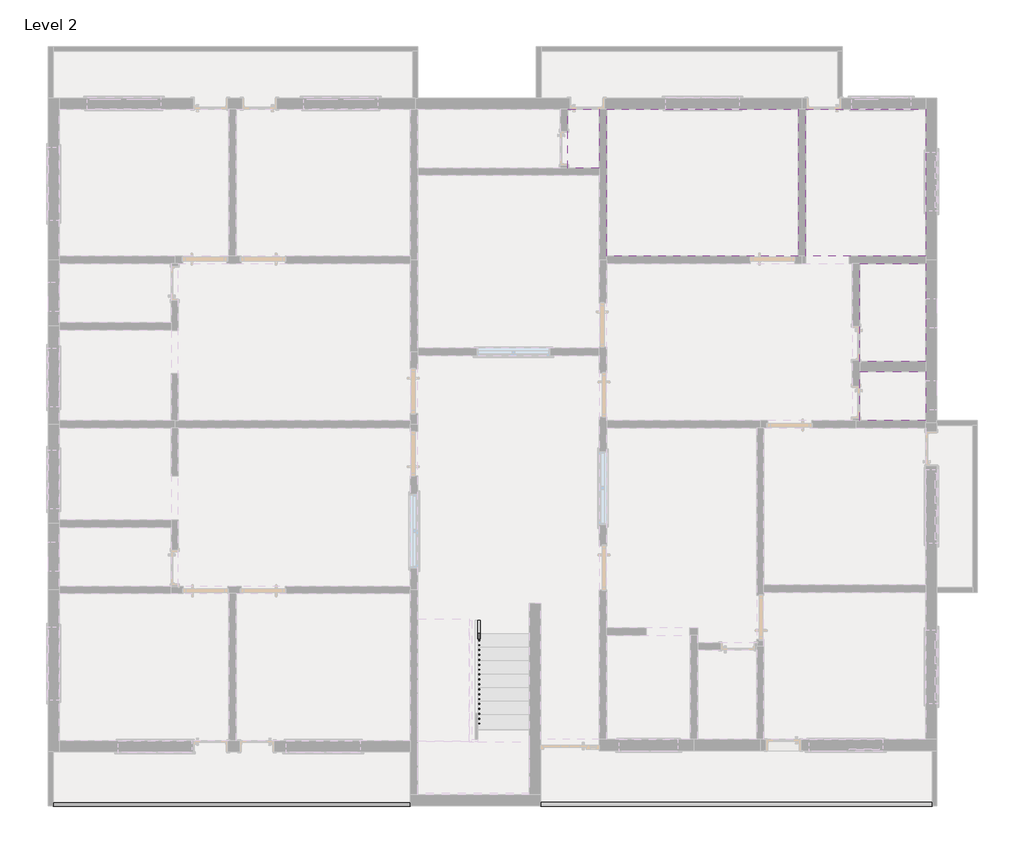
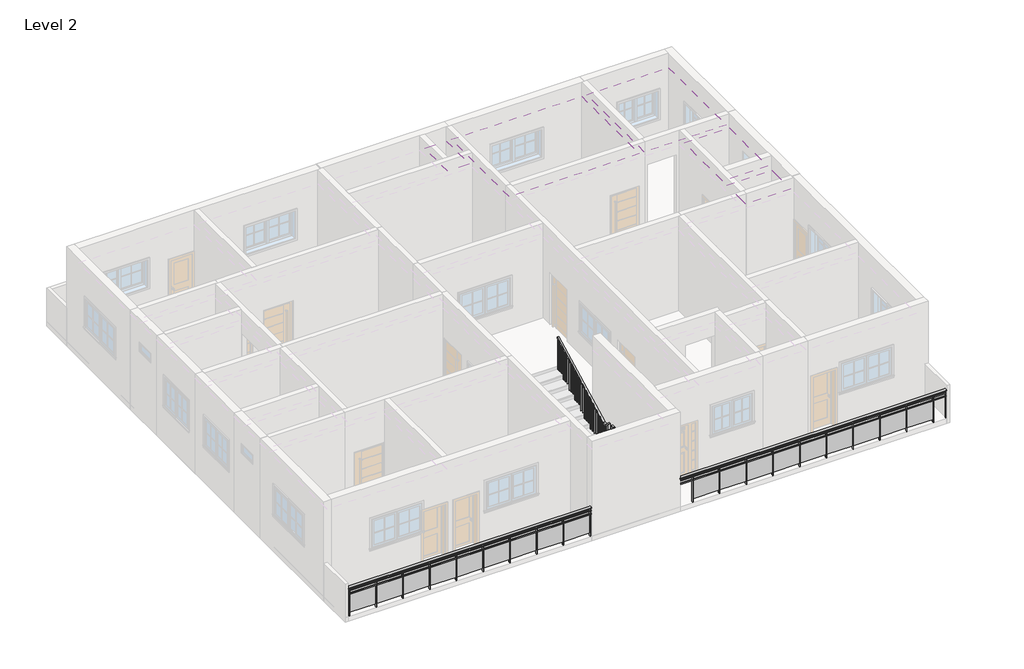
# One storey, part 4 of 5: 5 coverings, 3 railings.
"""IFC4 building model written with IfcOpenShell, lengths in millimetres."""

from ifc_helpers import new_model, si_unit, point, frame, origin, place, context, project, spatial, polyline, ellipse_curve, trimmed, outline, extrude, faceted_brep, element, save
from ifc_brep_helpers import plane_surface, extruded_surface, advanced_brep

model = new_model("IFC4")

# Units and contexts
model_context = context("Model", 3, world=origin())
ifc_project = project(units=[si_unit("LENGTHUNIT", "METRE", prefix="MILLI")], contexts=[model_context])

# Site, building, storey
site = spatial("IfcSite", under=ifc_project)
building = spatial("IfcBuilding", under=site)
storey = spatial("IfcBuildingStorey", under=building, Name="Level 2", Elevation=3200.4)

# Coverings
placement = place(None, origin())
element("IfcCovering", 1, ObjectType="2' x 4' ACT System", at=placement, inside=storey, context=model_context, shape_type="SweptSolid", body=[
    extrude(outline(polyline([(-9485.2847893, 20054.3922903), (-13447.6847893, 20054.3922903), (-13447.6847893, 23102.3922903), (-9485.2847893, 23102.3922903), (-9485.2847893, 20054.3922903)])), frame((0.0, 0.0, 5943.6), z_axis=(0.0, 0.0, 1.0), x_axis=(1.0, 0.0, 0.0)), (0.0, 0.0, 1.0), 57.15),
])
element("IfcCovering", 2, ObjectType="2' x 4' ACT System", at=placement, inside=storey, context=model_context, shape_type="SweptSolid", body=[
    extrude(outline(polyline([(-9332.8847893, 20054.3922903), (-9332.8847893, 23102.3922903), (-6843.6847893, 23102.3922903), (-6843.6847893, 20054.3922903), (-9332.8847893, 20054.3922903)])), frame((0.0, 0.0, 5943.6), z_axis=(0.0, 0.0, 1.0), x_axis=(1.0, 0.0, 0.0)), (0.0, 0.0, 1.0), 57.15),
])
element("IfcCovering", 3, ObjectType="2' x 4' ACT System", at=placement, inside=storey, context=model_context, shape_type="SweptSolid", body=[
    extrude(outline(polyline([(-6843.6847893, 17869.9922903), (-8215.2847893, 17869.9922903), (-8215.2847893, 19901.9922903), (-6843.6847893, 19901.9922903), (-6843.6847893, 17869.9922903)])), frame((0.0, 0.0, 5943.6), z_axis=(0.0, 0.0, 1.0), x_axis=(1.0, 0.0, 0.0)), (0.0, 0.0, 1.0), 57.15),
])
element("IfcCovering", 4, ObjectType="2' x 4' ACT System", at=placement, inside=storey, context=model_context, shape_type="SweptSolid", body=[
    extrude(outline(polyline([(-6843.6847893, 16650.7922903), (-8215.2847893, 16650.7922903), (-8215.2847893, 17666.7922903), (-6843.6847893, 17666.7922903), (-6843.6847893, 16650.7922903)])), frame((0.0, 0.0, 5943.6), z_axis=(0.0, 0.0, 1.0), x_axis=(1.0, 0.0, 0.0)), (0.0, 0.0, 1.0), 57.15),
])
element("IfcCovering", 5, ObjectType="2' x 4' ACT System", at=placement, inside=storey, context=model_context, shape_type="SweptSolid", body=[
    extrude(outline(polyline([(-14260.4847893, 23102.3922903), (-13600.0847893, 23102.3922903), (-13600.0847893, 21883.1922903), (-14260.4847893, 21883.1922903), (-14260.4847893, 23102.3922903)])), frame((0.0, 0.0, 5943.6), z_axis=(0.0, 0.0, 1.0), x_axis=(1.0, 0.0, 0.0)), (0.0, 0.0, 1.0), 57.15),
])

# Railings
element("IfcRailing", 6, ObjectType="Glass Panel - Bottom Fill", at=placement, inside=storey, context=model_context, shape_type="SolidModel", body=[
    advanced_brep(
    [(-24903.0847893, 8738.6922903, 4267.2), (-24903.0847893, 8662.4922903, 4267.2), (-17511.6847893, 8738.6922903, 4267.2), (-17511.6847893, 8662.4922903, 4267.2)],
    [
        (0, 1, ellipse_curve(frame((-24903.0847893, 8700.5922903, 4267.2), z_axis=(-1.0, 0.0, 0.0), x_axis=(0.0, -1.0, 0.0)), 38.1, 28.575)),
        (1, 0, ellipse_curve(frame((-24903.0847893, 8700.5922903, 4267.2), z_axis=(-1.0, 0.0, 0.0), x_axis=(0.0, -1.0, 0.0)), 38.1, 28.575)),
        (2, 3, ellipse_curve(frame((-17511.6847893, 8700.5922903, 4267.2), z_axis=(1.0, 0.0, 0.0), x_axis=(0.0, -1.0, 0.0)), 38.1, 28.575)),
        (3, 2, ellipse_curve(frame((-17511.6847893, 8700.5922903, 4267.2), z_axis=(1.0, 0.0, 0.0), x_axis=(0.0, -1.0, 0.0)), 38.1, 28.575)),
        (0, 2),
        (3, 1),
    ],
    [
        plane_surface(frame((-24903.0847893, 8700.5922903, 4267.2), z_axis=(-1.0, 0.0, 0.0), x_axis=(0.0, 1.0, 0.0))),
        plane_surface(frame((-17511.6847893, 8700.5922903, 4267.2), z_axis=(1.0, 0.0, 0.0), x_axis=(0.0, 1.0, 0.0))),
        extruded_surface(trimmed(ellipse_curve(frame((-17511.6847893, 8700.5922903, 4267.2), z_axis=(-1.0, 0.0, 0.0), x_axis=(0.0, -1.0, 0.0)), 38.1, 28.575), [point((-17511.6847893, 8738.6922903, 4267.2))], [point((-17511.6847893, 8662.4922903, 4267.2))], True, "CARTESIAN"), (-7391.399999999998, 0.0, 0.0), 7391.399999999998),
        extruded_surface(trimmed(ellipse_curve(frame((-17511.6847893, 8700.5922903, 4267.2), z_axis=(-1.0, 0.0, 0.0), x_axis=(0.0, -1.0, 0.0)), 38.1, 28.575), [point((-17511.6847893, 8662.4922903, 4267.2))], [point((-17511.6847893, 8738.6922903, 4267.2))], True, "CARTESIAN"), (-7391.399999999998, 0.0, 0.0), 7391.399999999998),
    ],
    [
        (0, [[1, 2]]),
        (1, [[3, 4]]),
        (2, [[-1, 5, -4, 6]]),
        (3, [[-2, -6, -3, -5]]),
    ],
),
    extrude(outline(polyline([(-24903.0847893, 8687.8922903), (-24903.0847893, 8713.2922903), (-17511.6847893, 8713.2922903), (-17511.6847893, 8687.8922903), (-24903.0847893, 8687.8922903)])), frame((0.0, 0.0, 4152.9), z_axis=(0.0, 0.0, 1.0), x_axis=(1.0, 0.0, 0.0)), (0.0, 0.0, 1.0), 25.4),
    extrude(outline(polyline([(-24903.0847893, 8687.8922903), (-24903.0847893, 8713.2922903), (-17511.6847893, 8713.2922903), (-17511.6847893, 8687.8922903), (-24903.0847893, 8687.8922903)])), frame((0.0, 0.0, 4051.3), z_axis=(0.0, 0.0, 1.0), x_axis=(1.0, 0.0, 0.0)), (0.0, 0.0, 1.0), 25.4),
    extrude(outline(polyline([(-17556.1347893, 8675.1922903), (-17556.1347893, 8725.9922903), (-17543.4347893, 8725.9922903), (-17543.4347893, 8675.1922903), (-17556.1347893, 8675.1922903)])), frame((0.0, 0.0, 3352.8), z_axis=(0.0, 0.0, 1.0), x_axis=(1.0, 0.0, 0.0)), (0.0, 0.0, 1.0), 885.825),
    extrude(outline(polyline([(-18362.5847893, 8707.1274473), (-17549.7847893, 8707.1274473), (-17549.7847893, 8700.7774473), (-18362.5847893, 8700.7774473), (-18362.5847893, 8707.1274473)])), frame((0.0, 0.0, 3454.4), z_axis=(0.0, 0.0, 1.0), x_axis=(1.0, 0.0, 0.0)), (0.0, 0.0, 1.0), 596.9),
    extrude(outline(polyline([(-18368.9347893, 8675.1922903), (-18368.9347893, 8725.9922903), (-18356.2347893, 8725.9922903), (-18356.2347893, 8675.1922903), (-18368.9347893, 8675.1922903)])), frame((0.0, 0.0, 3352.8), z_axis=(0.0, 0.0, 1.0), x_axis=(1.0, 0.0, 0.0)), (0.0, 0.0, 1.0), 885.825),
    extrude(outline(polyline([(-19175.3847893, 8707.1274473), (-18362.5847893, 8707.1274473), (-18362.5847893, 8700.7774473), (-19175.3847893, 8700.7774473), (-19175.3847893, 8707.1274473)])), frame((0.0, 0.0, 3454.4), z_axis=(0.0, 0.0, 1.0), x_axis=(1.0, 0.0, 0.0)), (0.0, 0.0, 1.0), 596.9),
    extrude(outline(polyline([(-19181.7347893, 8675.1922903), (-19181.7347893, 8725.9922903), (-19169.0347893, 8725.9922903), (-19169.0347893, 8675.1922903), (-19181.7347893, 8675.1922903)])), frame((0.0, 0.0, 3352.8), z_axis=(0.0, 0.0, 1.0), x_axis=(1.0, 0.0, 0.0)), (0.0, 0.0, 1.0), 885.825),
    extrude(outline(polyline([(-19988.1847893, 8707.1274473), (-19175.3847893, 8707.1274473), (-19175.3847893, 8700.7774473), (-19988.1847893, 8700.7774473), (-19988.1847893, 8707.1274473)])), frame((0.0, 0.0, 3454.4), z_axis=(0.0, 0.0, 1.0), x_axis=(1.0, 0.0, 0.0)), (0.0, 0.0, 1.0), 596.9),
    extrude(outline(polyline([(-19994.5347893, 8675.1922903), (-19994.5347893, 8725.9922903), (-19981.8347893, 8725.9922903), (-19981.8347893, 8675.1922903), (-19994.5347893, 8675.1922903)])), frame((0.0, 0.0, 3352.8), z_axis=(0.0, 0.0, 1.0), x_axis=(1.0, 0.0, 0.0)), (0.0, 0.0, 1.0), 885.825),
    extrude(outline(polyline([(-20800.9847893, 8707.1274473), (-19988.1847893, 8707.1274473), (-19988.1847893, 8700.7774473), (-20800.9847893, 8700.7774473), (-20800.9847893, 8707.1274473)])), frame((0.0, 0.0, 3454.4), z_axis=(0.0, 0.0, 1.0), x_axis=(1.0, 0.0, 0.0)), (0.0, 0.0, 1.0), 596.9),
    extrude(outline(polyline([(-20807.3347893, 8675.1922903), (-20807.3347893, 8725.9922903), (-20794.6347893, 8725.9922903), (-20794.6347893, 8675.1922903), (-20807.3347893, 8675.1922903)])), frame((0.0, 0.0, 3352.8), z_axis=(0.0, 0.0, 1.0), x_axis=(1.0, 0.0, 0.0)), (0.0, 0.0, 1.0), 885.825),
    extrude(outline(polyline([(-21613.7847893, 8707.1274473), (-20800.9847893, 8707.1274473), (-20800.9847893, 8700.7774473), (-21613.7847893, 8700.7774473), (-21613.7847893, 8707.1274473)])), frame((0.0, 0.0, 3454.4), z_axis=(0.0, 0.0, 1.0), x_axis=(1.0, 0.0, 0.0)), (0.0, 0.0, 1.0), 596.9),
    extrude(outline(polyline([(-21620.1347893, 8675.1922903), (-21620.1347893, 8725.9922903), (-21607.4347893, 8725.9922903), (-21607.4347893, 8675.1922903), (-21620.1347893, 8675.1922903)])), frame((0.0, 0.0, 3352.8), z_axis=(0.0, 0.0, 1.0), x_axis=(1.0, 0.0, 0.0)), (0.0, 0.0, 1.0), 885.825),
    extrude(outline(polyline([(-22426.5847893, 8707.1274473), (-21613.7847893, 8707.1274473), (-21613.7847893, 8700.7774473), (-22426.5847893, 8700.7774473), (-22426.5847893, 8707.1274473)])), frame((0.0, 0.0, 3454.4), z_axis=(0.0, 0.0, 1.0), x_axis=(1.0, 0.0, 0.0)), (0.0, 0.0, 1.0), 596.9),
    extrude(outline(polyline([(-22432.9347893, 8675.1922903), (-22432.9347893, 8725.9922903), (-22420.2347893, 8725.9922903), (-22420.2347893, 8675.1922903), (-22432.9347893, 8675.1922903)])), frame((0.0, 0.0, 3352.8), z_axis=(0.0, 0.0, 1.0), x_axis=(1.0, 0.0, 0.0)), (0.0, 0.0, 1.0), 885.825),
    extrude(outline(polyline([(-23239.3847893, 8707.1274473), (-22426.5847893, 8707.1274473), (-22426.5847893, 8700.7774473), (-23239.3847893, 8700.7774473), (-23239.3847893, 8707.1274473)])), frame((0.0, 0.0, 3454.4), z_axis=(0.0, 0.0, 1.0), x_axis=(1.0, 0.0, 0.0)), (0.0, 0.0, 1.0), 596.9),
    extrude(outline(polyline([(-23245.7347893, 8675.1922903), (-23245.7347893, 8725.9922903), (-23233.0347893, 8725.9922903), (-23233.0347893, 8675.1922903), (-23245.7347893, 8675.1922903)])), frame((0.0, 0.0, 3352.8), z_axis=(0.0, 0.0, 1.0), x_axis=(1.0, 0.0, 0.0)), (0.0, 0.0, 1.0), 885.825),
    extrude(outline(polyline([(-24052.1847893, 8707.1274473), (-23239.3847893, 8707.1274473), (-23239.3847893, 8700.7774473), (-24052.1847893, 8700.7774473), (-24052.1847893, 8707.1274473)])), frame((0.0, 0.0, 3454.4), z_axis=(0.0, 0.0, 1.0), x_axis=(1.0, 0.0, 0.0)), (0.0, 0.0, 1.0), 596.9),
    extrude(outline(polyline([(-24058.5347893, 8675.1922903), (-24058.5347893, 8725.9922903), (-24045.8347893, 8725.9922903), (-24045.8347893, 8675.1922903), (-24058.5347893, 8675.1922903)])), frame((0.0, 0.0, 3352.8), z_axis=(0.0, 0.0, 1.0), x_axis=(1.0, 0.0, 0.0)), (0.0, 0.0, 1.0), 885.825),
    extrude(outline(polyline([(-24864.9847893, 8707.1274473), (-24052.1847893, 8707.1274473), (-24052.1847893, 8700.7774473), (-24864.9847893, 8700.7774473), (-24864.9847893, 8707.1274473)])), frame((0.0, 0.0, 3454.4), z_axis=(0.0, 0.0, 1.0), x_axis=(1.0, 0.0, 0.0)), (0.0, 0.0, 1.0), 596.9),
    extrude(outline(polyline([(-24871.3347893, 8675.1922903), (-24871.3347893, 8725.9922903), (-24858.6347893, 8725.9922903), (-24858.6347893, 8675.1922903), (-24871.3347893, 8675.1922903)])), frame((0.0, 0.0, 3352.8), z_axis=(0.0, 0.0, 1.0), x_axis=(1.0, 0.0, 0.0)), (0.0, 0.0, 1.0), 885.825),
    extrude(outline(polyline([(-17524.3847893, 8691.0672903), (-17524.3847893, 8710.1172903), (-17505.3347893, 8710.1172903), (-17505.3347893, 8691.0672903), (-17524.3847893, 8691.0672903)])), frame((0.0, 0.0, 3352.8), z_axis=(0.0, 0.0, 1.0), x_axis=(1.0, 0.0, 0.0)), (0.0, 0.0, 1.0), 885.825),
    extrude(outline(polyline([(-24909.4347893, 8691.0672903), (-24909.4347893, 8710.1172903), (-24890.3847893, 8710.1172903), (-24890.3847893, 8691.0672903), (-24909.4347893, 8691.0672903)])), frame((0.0, 0.0, 3352.8), z_axis=(0.0, 0.0, 1.0), x_axis=(1.0, 0.0, 0.0)), (0.0, 0.0, 1.0), 885.825),
])
element("IfcRailing", 7, ObjectType="Glass Panel - Bottom Fill", at=placement, inside=storey, context=model_context, shape_type="SolidModel", body=[
    advanced_brep(
    [(-6716.6847893, 8668.8422903, 4267.2), (-6716.6847893, 8745.0422903, 4267.2), (-14819.2847893, 8668.8422903, 4267.2), (-14819.2847893, 8745.0422903, 4267.2)],
    [
        (0, 1, ellipse_curve(frame((-6716.6847893, 8706.9422903, 4267.2), z_axis=(1.0, 0.0, 0.0), x_axis=(0.0, 1.0, 0.0)), 38.1, 28.575)),
        (1, 0, ellipse_curve(frame((-6716.6847893, 8706.9422903, 4267.2), z_axis=(1.0, 0.0, 0.0), x_axis=(0.0, 1.0, 0.0)), 38.1, 28.575)),
        (2, 3, ellipse_curve(frame((-14819.2847893, 8706.9422903, 4267.2), z_axis=(-1.0, 0.0, 0.0), x_axis=(0.0, 1.0, 0.0)), 38.1, 28.575)),
        (3, 2, ellipse_curve(frame((-14819.2847893, 8706.9422903, 4267.2), z_axis=(-1.0, 0.0, 0.0), x_axis=(0.0, 1.0, 0.0)), 38.1, 28.575)),
        (0, 2),
        (3, 1),
    ],
    [
        plane_surface(frame((-6716.6847893, 8706.9422903, 4267.2), z_axis=(1.0, 0.0, 0.0), x_axis=(0.0, -1.0, 0.0))),
        plane_surface(frame((-14819.2847893, 8706.9422903, 4267.2), z_axis=(-1.0, 0.0, 0.0), x_axis=(0.0, -1.0, 0.0))),
        extruded_surface(trimmed(ellipse_curve(frame((-14819.2847893, 8706.9422903, 4267.2), z_axis=(1.0, 0.0, 0.0), x_axis=(0.0, 1.0, 0.0)), 38.1, 28.575), [point((-14819.2847893, 8668.8422903, 4267.2))], [point((-14819.2847893, 8745.0422903, 4267.2))], True, "CARTESIAN"), (8102.599999999999, 0.0, 0.0), 8102.599999999999),
        extruded_surface(trimmed(ellipse_curve(frame((-14819.2847893, 8706.9422903, 4267.2), z_axis=(1.0, 0.0, 0.0), x_axis=(0.0, 1.0, 0.0)), 38.1, 28.575), [point((-14819.2847893, 8745.0422903, 4267.2))], [point((-14819.2847893, 8668.8422903, 4267.2))], True, "CARTESIAN"), (8102.599999999999, 0.0, 0.0), 8102.599999999999),
    ],
    [
        (0, [[1, 2]]),
        (1, [[3, 4]]),
        (2, [[-1, 5, -4, 6]]),
        (3, [[-2, -6, -3, -5]]),
    ],
),
    extrude(outline(polyline([(-6716.6847893, 8719.6422903), (-6716.6847893, 8694.2422903), (-14819.2847893, 8694.2422903), (-14819.2847893, 8719.6422903), (-6716.6847893, 8719.6422903)])), frame((0.0, 0.0, 4152.9), z_axis=(0.0, 0.0, 1.0), x_axis=(1.0, 0.0, 0.0)), (0.0, 0.0, 1.0), 25.4),
    extrude(outline(polyline([(-6716.6847893, 8719.6422903), (-6716.6847893, 8694.2422903), (-14819.2847893, 8694.2422903), (-14819.2847893, 8719.6422903), (-6716.6847893, 8719.6422903)])), frame((0.0, 0.0, 4051.3), z_axis=(0.0, 0.0, 1.0), x_axis=(1.0, 0.0, 0.0)), (0.0, 0.0, 1.0), 25.4),
    extrude(outline(polyline([(-14419.2347893, 8732.3422903), (-14419.2347893, 8681.5422903), (-14431.9347893, 8681.5422903), (-14431.9347893, 8732.3422903), (-14419.2347893, 8732.3422903)])), frame((0.0, 0.0, 3352.8), z_axis=(0.0, 0.0, 1.0), x_axis=(1.0, 0.0, 0.0)), (0.0, 0.0, 1.0), 885.825),
    extrude(outline(polyline([(-13612.7847893, 8700.4071333), (-14425.5847893, 8700.4071333), (-14425.5847893, 8706.7571333), (-13612.7847893, 8706.7571333), (-13612.7847893, 8700.4071333)])), frame((0.0, 0.0, 3454.4), z_axis=(0.0, 0.0, 1.0), x_axis=(1.0, 0.0, 0.0)), (0.0, 0.0, 1.0), 596.9),
    extrude(outline(polyline([(-13606.4347893, 8732.3422903), (-13606.4347893, 8681.5422903), (-13619.1347893, 8681.5422903), (-13619.1347893, 8732.3422903), (-13606.4347893, 8732.3422903)])), frame((0.0, 0.0, 3352.8), z_axis=(0.0, 0.0, 1.0), x_axis=(1.0, 0.0, 0.0)), (0.0, 0.0, 1.0), 885.825),
    extrude(outline(polyline([(-12799.9847893, 8700.4071333), (-13612.7847893, 8700.4071333), (-13612.7847893, 8706.7571333), (-12799.9847893, 8706.7571333), (-12799.9847893, 8700.4071333)])), frame((0.0, 0.0, 3454.4), z_axis=(0.0, 0.0, 1.0), x_axis=(1.0, 0.0, 0.0)), (0.0, 0.0, 1.0), 596.9),
    extrude(outline(polyline([(-12793.6347893, 8732.3422903), (-12793.6347893, 8681.5422903), (-12806.3347893, 8681.5422903), (-12806.3347893, 8732.3422903), (-12793.6347893, 8732.3422903)])), frame((0.0, 0.0, 3352.8), z_axis=(0.0, 0.0, 1.0), x_axis=(1.0, 0.0, 0.0)), (0.0, 0.0, 1.0), 885.825),
    extrude(outline(polyline([(-11987.1847893, 8700.4071333), (-12799.9847893, 8700.4071333), (-12799.9847893, 8706.7571333), (-11987.1847893, 8706.7571333), (-11987.1847893, 8700.4071333)])), frame((0.0, 0.0, 3454.4), z_axis=(0.0, 0.0, 1.0), x_axis=(1.0, 0.0, 0.0)), (0.0, 0.0, 1.0), 596.9),
    extrude(outline(polyline([(-11980.8347893, 8732.3422903), (-11980.8347893, 8681.5422903), (-11993.5347893, 8681.5422903), (-11993.5347893, 8732.3422903), (-11980.8347893, 8732.3422903)])), frame((0.0, 0.0, 3352.8), z_axis=(0.0, 0.0, 1.0), x_axis=(1.0, 0.0, 0.0)), (0.0, 0.0, 1.0), 885.825),
    extrude(outline(polyline([(-11174.3847893, 8700.4071333), (-11987.1847893, 8700.4071333), (-11987.1847893, 8706.7571333), (-11174.3847893, 8706.7571333), (-11174.3847893, 8700.4071333)])), frame((0.0, 0.0, 3454.4), z_axis=(0.0, 0.0, 1.0), x_axis=(1.0, 0.0, 0.0)), (0.0, 0.0, 1.0), 596.9),
    extrude(outline(polyline([(-11168.0347893, 8732.3422903), (-11168.0347893, 8681.5422903), (-11180.7347893, 8681.5422903), (-11180.7347893, 8732.3422903), (-11168.0347893, 8732.3422903)])), frame((0.0, 0.0, 3352.8), z_axis=(0.0, 0.0, 1.0), x_axis=(1.0, 0.0, 0.0)), (0.0, 0.0, 1.0), 885.825),
    extrude(outline(polyline([(-10361.5847893, 8700.4071333), (-11174.3847893, 8700.4071333), (-11174.3847893, 8706.7571333), (-10361.5847893, 8706.7571333), (-10361.5847893, 8700.4071333)])), frame((0.0, 0.0, 3454.4), z_axis=(0.0, 0.0, 1.0), x_axis=(1.0, 0.0, 0.0)), (0.0, 0.0, 1.0), 596.9),
    extrude(outline(polyline([(-10355.2347893, 8732.3422903), (-10355.2347893, 8681.5422903), (-10367.9347893, 8681.5422903), (-10367.9347893, 8732.3422903), (-10355.2347893, 8732.3422903)])), frame((0.0, 0.0, 3352.8), z_axis=(0.0, 0.0, 1.0), x_axis=(1.0, 0.0, 0.0)), (0.0, 0.0, 1.0), 885.825),
    extrude(outline(polyline([(-9548.7847893, 8700.4071333), (-10361.5847893, 8700.4071333), (-10361.5847893, 8706.7571333), (-9548.7847893, 8706.7571333), (-9548.7847893, 8700.4071333)])), frame((0.0, 0.0, 3454.4), z_axis=(0.0, 0.0, 1.0), x_axis=(1.0, 0.0, 0.0)), (0.0, 0.0, 1.0), 596.9),
    extrude(outline(polyline([(-9542.4347893, 8732.3422903), (-9542.4347893, 8681.5422903), (-9555.1347893, 8681.5422903), (-9555.1347893, 8732.3422903), (-9542.4347893, 8732.3422903)])), frame((0.0, 0.0, 3352.8), z_axis=(0.0, 0.0, 1.0), x_axis=(1.0, 0.0, 0.0)), (0.0, 0.0, 1.0), 885.825),
    extrude(outline(polyline([(-8735.9847893, 8700.4071333), (-9548.7847893, 8700.4071333), (-9548.7847893, 8706.7571333), (-8735.9847893, 8706.7571333), (-8735.9847893, 8700.4071333)])), frame((0.0, 0.0, 3454.4), z_axis=(0.0, 0.0, 1.0), x_axis=(1.0, 0.0, 0.0)), (0.0, 0.0, 1.0), 596.9),
    extrude(outline(polyline([(-8729.6347893, 8732.3422903), (-8729.6347893, 8681.5422903), (-8742.3347893, 8681.5422903), (-8742.3347893, 8732.3422903), (-8729.6347893, 8732.3422903)])), frame((0.0, 0.0, 3352.8), z_axis=(0.0, 0.0, 1.0), x_axis=(1.0, 0.0, 0.0)), (0.0, 0.0, 1.0), 885.825),
    extrude(outline(polyline([(-7923.1847893, 8700.4071333), (-8735.9847893, 8700.4071333), (-8735.9847893, 8706.7571333), (-7923.1847893, 8706.7571333), (-7923.1847893, 8700.4071333)])), frame((0.0, 0.0, 3454.4), z_axis=(0.0, 0.0, 1.0), x_axis=(1.0, 0.0, 0.0)), (0.0, 0.0, 1.0), 596.9),
    extrude(outline(polyline([(-7916.8347893, 8732.3422903), (-7916.8347893, 8681.5422903), (-7929.5347893, 8681.5422903), (-7929.5347893, 8732.3422903), (-7916.8347893, 8732.3422903)])), frame((0.0, 0.0, 3352.8), z_axis=(0.0, 0.0, 1.0), x_axis=(1.0, 0.0, 0.0)), (0.0, 0.0, 1.0), 885.825),
    extrude(outline(polyline([(-7110.3847893, 8700.4071333), (-7923.1847893, 8700.4071333), (-7923.1847893, 8706.7571333), (-7110.3847893, 8706.7571333), (-7110.3847893, 8700.4071333)])), frame((0.0, 0.0, 3454.4), z_axis=(0.0, 0.0, 1.0), x_axis=(1.0, 0.0, 0.0)), (0.0, 0.0, 1.0), 596.9),
    extrude(outline(polyline([(-7104.0347893, 8732.3422903), (-7104.0347893, 8681.5422903), (-7116.7347893, 8681.5422903), (-7116.7347893, 8732.3422903), (-7104.0347893, 8732.3422903)])), frame((0.0, 0.0, 3352.8), z_axis=(0.0, 0.0, 1.0), x_axis=(1.0, 0.0, 0.0)), (0.0, 0.0, 1.0), 885.825),
    extrude(outline(polyline([(-14806.5847893, 8716.4672903), (-14806.5847893, 8697.4172903), (-14825.6347893, 8697.4172903), (-14825.6347893, 8716.4672903), (-14806.5847893, 8716.4672903)])), frame((0.0, 0.0, 3352.8), z_axis=(0.0, 0.0, 1.0), x_axis=(1.0, 0.0, 0.0)), (0.0, 0.0, 1.0), 885.825),
    extrude(outline(polyline([(-6710.3347893, 8716.4672903), (-6710.3347893, 8697.4172903), (-6729.3847893, 8697.4172903), (-6729.3847893, 8716.4672903), (-6710.3347893, 8716.4672903)])), frame((0.0, 0.0, 3352.8), z_axis=(0.0, 0.0, 1.0), x_axis=(1.0, 0.0, 0.0)), (0.0, 0.0, 1.0), 885.825),
])
element("IfcRailing", 8, ObjectType="Handrail - Rectangular", at=placement, inside=storey, context=model_context, shape_type="SolidModel", body=[
    faceted_brep([(-16063.8847893, 12510.5922903, 4260.2727273), (-16063.8847893, 12510.5922903, 4202.9995168), (-16114.6847893, 12510.5922903, 4202.9995168), (-16114.6847893, 12510.5922903, 4260.2727273), (-16063.8847893, 10072.1922903, 5529.8528926), (-16063.8847893, 10021.3922903, 5499.0292688), (-16114.6847893, 10021.3922903, 5499.0292688), (-16114.6847893, 10072.1922903, 5529.8528926), (-16063.8847893, 10072.1922903, 5569.5272727), (-16063.8847893, 10021.3922903, 5518.7272727), (-16114.6847893, 10021.3922903, 5518.7272727), (-16114.6847893, 10072.1922903, 5569.5272727), (-16063.8847893, 9945.1922903, 5569.5272727), (-16063.8847893, 9945.1922903, 5518.7272727), (-16114.6847893, 9995.9922903, 5518.7272727), (-16114.6847893, 9995.9922903, 5569.5272727), (-16190.8847893, 9945.1922903, 5569.5272727), (-16190.8847893, 9945.1922903, 5518.7272727), (-16190.8847893, 9995.9922903, 5518.7272727), (-16190.8847893, 9995.9922903, 5569.5272727), (-16216.2847893, 9945.1922903, 5569.5272727), (-16267.0847893, 9945.1922903, 5518.7272727), (-16267.0847893, 9995.9922903, 5518.7272727), (-16216.2847893, 9995.9922903, 5569.5272727), (-16216.2847893, 9945.1922903, 5754.6743802), (-16267.0847893, 9945.1922903, 5703.8743802), (-16267.0847893, 9995.9922903, 5703.8743802), (-16216.2847893, 9995.9922903, 5754.6743802), (-16343.2847893, 9945.1922903, 5754.6743802), (-16343.2847893, 9945.1922903, 5703.8743802), (-16292.4847893, 9995.9922903, 5703.8743802), (-16292.4847893, 9995.9922903, 5754.6743802), (-16343.2847893, 10072.1922903, 5754.6743802), (-16343.2847893, 10084.6249644, 5703.8743802), (-16292.4847893, 10084.6249644, 5703.8743802), (-16292.4847893, 10072.1922903, 5754.6743802), (-16343.2847893, 12510.5922903, 7024.2545455), (-16292.4847893, 12510.5922903, 7024.2545455), (-16292.4847893, 12510.5922903, 6966.981335), (-16343.2847893, 12510.5922903, 6966.981335)], [[[0, 1, 2, 3]], [[1, 0, 4, 5]], [[2, 1, 5, 6]], [[3, 2, 6, 7]], [[0, 3, 7, 4]], [[5, 4, 8, 9]], [[6, 5, 9, 10]], [[7, 6, 10, 11]], [[4, 7, 11, 8]], [[9, 8, 12, 13]], [[10, 9, 13, 14]], [[11, 10, 14, 15]], [[8, 11, 15, 12]], [[13, 12, 16, 17]], [[14, 13, 17, 18]], [[15, 14, 18, 19]], [[12, 15, 19, 16]], [[17, 16, 20, 21]], [[18, 17, 21, 22]], [[19, 18, 22, 23]], [[16, 19, 23, 20]], [[21, 20, 24, 25]], [[22, 21, 25, 26]], [[23, 22, 26, 27]], [[20, 23, 27, 24]], [[25, 24, 28, 29]], [[26, 25, 29, 30]], [[27, 26, 30, 31]], [[24, 27, 31, 28]], [[29, 28, 32, 33]], [[30, 29, 33, 34]], [[31, 30, 34, 35]], [[28, 31, 35, 32]], [[36, 37, 38, 39]], [[33, 32, 36, 39]], [[34, 33, 39, 38]], [[35, 34, 38, 37]], [[32, 35, 37, 36]]]),
    extrude(outline(polyline([(12399.4672903, 6909.1228639), (12418.5172903, 6919.0414589), (12418.5172903, 5964.3818182), (12399.4672903, 5964.3818182), (12399.4672903, 6909.1228639)])), frame((-16327.4097893, 0.0, 0.0), z_axis=(1.0, 0.0, 0.0), x_axis=(0.0, 1.0, 0.0)), (0.0, 0.0, 1.0), 19.05),
    extrude(outline(polyline([(12297.8672903, 6856.2236903), (12316.9172903, 6866.1422854), (12316.9172903, 5964.3818182), (12297.8672903, 5964.3818182), (12297.8672903, 6856.2236903)])), frame((-16327.4097893, 0.0, 0.0), z_axis=(1.0, 0.0, 0.0), x_axis=(0.0, 1.0, 0.0)), (0.0, 0.0, 1.0), 19.05),
    extrude(outline(polyline([(12196.2672903, 6803.3245168), (12215.3172903, 6813.2431118), (12215.3172903, 5818.9090909), (12196.2672903, 5818.9090909), (12196.2672903, 6803.3245168)])), frame((-16327.4097893, 0.0, 0.0), z_axis=(1.0, 0.0, 0.0), x_axis=(0.0, 1.0, 0.0)), (0.0, 0.0, 1.0), 19.05),
    extrude(outline(polyline([(12094.6672903, 6750.4253432), (12113.7172903, 6760.3439383), (12113.7172903, 5818.9090909), (12094.6672903, 5818.9090909), (12094.6672903, 6750.4253432)])), frame((-16327.4097893, 0.0, 0.0), z_axis=(1.0, 0.0, 0.0), x_axis=(0.0, 1.0, 0.0)), (0.0, 0.0, 1.0), 19.05),
    extrude(outline(polyline([(11993.0672903, 6697.5261697), (12012.1172903, 6707.4447647), (12012.1172903, 5818.9090909), (11993.0672903, 5818.9090909), (11993.0672903, 6697.5261697)])), frame((-16327.4097893, 0.0, 0.0), z_axis=(1.0, 0.0, 0.0), x_axis=(0.0, 1.0, 0.0)), (0.0, 0.0, 1.0), 19.05),
    extrude(outline(polyline([(11891.4672903, 6644.6269961), (11910.5172903, 6654.5455912), (11910.5172903, 5673.4363636), (11891.4672903, 5673.4363636), (11891.4672903, 6644.6269961)])), frame((-16327.4097893, 0.0, 0.0), z_axis=(1.0, 0.0, 0.0), x_axis=(0.0, 1.0, 0.0)), (0.0, 0.0, 1.0), 19.05),
    extrude(outline(polyline([(11789.8672903, 6591.7278226), (11808.9172903, 6601.6464176), (11808.9172903, 5673.4363636), (11789.8672903, 5673.4363636), (11789.8672903, 6591.7278226)])), frame((-16327.4097893, 0.0, 0.0), z_axis=(1.0, 0.0, 0.0), x_axis=(0.0, 1.0, 0.0)), (0.0, 0.0, 1.0), 19.05),
    extrude(outline(polyline([(11688.2672903, 6538.828649), (11707.3172903, 6548.747244), (11707.3172903, 5673.4363636), (11688.2672903, 5673.4363636), (11688.2672903, 6538.828649)])), frame((-16327.4097893, 0.0, 0.0), z_axis=(1.0, 0.0, 0.0), x_axis=(0.0, 1.0, 0.0)), (0.0, 0.0, 1.0), 19.05),
    extrude(outline(polyline([(11586.6672903, 6485.9294755), (11605.7172903, 6495.8480705), (11605.7172903, 5527.9636364), (11586.6672903, 5527.9636364), (11586.6672903, 6485.9294755)])), frame((-16327.4097893, 0.0, 0.0), z_axis=(1.0, 0.0, 0.0), x_axis=(0.0, 1.0, 0.0)), (0.0, 0.0, 1.0), 19.05),
    extrude(outline(polyline([(11485.0672903, 6433.0303019), (11504.1172903, 6442.9488969), (11504.1172903, 5527.9636364), (11485.0672903, 5527.9636364), (11485.0672903, 6433.0303019)])), frame((-16327.4097893, 0.0, 0.0), z_axis=(1.0, 0.0, 0.0), x_axis=(0.0, 1.0, 0.0)), (0.0, 0.0, 1.0), 19.05),
    extrude(outline(polyline([(11383.4672903, 6380.1311283), (11402.5172903, 6390.0497234), (11402.5172903, 5527.9636364), (11383.4672903, 5527.9636364), (11383.4672903, 6380.1311283)])), frame((-16327.4097893, 0.0, 0.0), z_axis=(1.0, 0.0, 0.0), x_axis=(0.0, 1.0, 0.0)), (0.0, 0.0, 1.0), 19.05),
    extrude(outline(polyline([(11281.8672903, 6327.2319548), (11300.9172903, 6337.1505498), (11300.9172903, 5382.4909091), (11281.8672903, 5382.4909091), (11281.8672903, 6327.2319548)])), frame((-16327.4097893, 0.0, 0.0), z_axis=(1.0, 0.0, 0.0), x_axis=(0.0, 1.0, 0.0)), (0.0, 0.0, 1.0), 19.05),
    extrude(outline(polyline([(11180.2672903, 6274.3327812), (11199.3172903, 6284.2513763), (11199.3172903, 5382.4909091), (11180.2672903, 5382.4909091), (11180.2672903, 6274.3327812)])), frame((-16327.4097893, 0.0, 0.0), z_axis=(1.0, 0.0, 0.0), x_axis=(0.0, 1.0, 0.0)), (0.0, 0.0, 1.0), 19.05),
    extrude(outline(polyline([(11078.6672903, 6221.4336077), (11097.7172903, 6231.3522027), (11097.7172903, 5237.0181818), (11078.6672903, 5237.0181818), (11078.6672903, 6221.4336077)])), frame((-16327.4097893, 0.0, 0.0), z_axis=(1.0, 0.0, 0.0), x_axis=(0.0, 1.0, 0.0)), (0.0, 0.0, 1.0), 19.05),
    extrude(outline(polyline([(10977.0672903, 6168.5344341), (10996.1172903, 6178.4530292), (10996.1172903, 5237.0181818), (10977.0672903, 5237.0181818), (10977.0672903, 6168.5344341)])), frame((-16327.4097893, 0.0, 0.0), z_axis=(1.0, 0.0, 0.0), x_axis=(0.0, 1.0, 0.0)), (0.0, 0.0, 1.0), 19.05),
    extrude(outline(polyline([(10875.4672903, 6115.6352606), (10894.5172903, 6125.5538556), (10894.5172903, 5237.0181818), (10875.4672903, 5237.0181818), (10875.4672903, 6115.6352606)])), frame((-16327.4097893, 0.0, 0.0), z_axis=(1.0, 0.0, 0.0), x_axis=(0.0, 1.0, 0.0)), (0.0, 0.0, 1.0), 19.05),
    extrude(outline(polyline([(10773.8672903, 6062.736087), (10792.9172903, 6072.6546821), (10792.9172903, 5091.5454545), (10773.8672903, 5091.5454545), (10773.8672903, 6062.736087)])), frame((-16327.4097893, 0.0, 0.0), z_axis=(1.0, 0.0, 0.0), x_axis=(0.0, 1.0, 0.0)), (0.0, 0.0, 1.0), 19.05),
    extrude(outline(polyline([(10672.2672903, 6009.8369135), (10691.3172903, 6019.7555085), (10691.3172903, 5091.5454545), (10672.2672903, 5091.5454545), (10672.2672903, 6009.8369135)])), frame((-16327.4097893, 0.0, 0.0), z_axis=(1.0, 0.0, 0.0), x_axis=(0.0, 1.0, 0.0)), (0.0, 0.0, 1.0), 19.05),
    extrude(outline(polyline([(10570.6672903, 5956.9377399), (10589.7172903, 5966.856335), (10589.7172903, 5091.5454545), (10570.6672903, 5091.5454545), (10570.6672903, 5956.9377399)])), frame((-16327.4097893, 0.0, 0.0), z_axis=(1.0, 0.0, 0.0), x_axis=(0.0, 1.0, 0.0)), (0.0, 0.0, 1.0), 19.05),
    extrude(outline(polyline([(10469.0672903, 5904.0385664), (10488.1172903, 5913.9571614), (10488.1172903, 4946.0727273), (10469.0672903, 4946.0727273), (10469.0672903, 5904.0385664)])), frame((-16327.4097893, 0.0, 0.0), z_axis=(1.0, 0.0, 0.0), x_axis=(0.0, 1.0, 0.0)), (0.0, 0.0, 1.0), 19.05),
    extrude(outline(polyline([(10367.4672903, 5851.1393928), (10386.5172903, 5861.0579878), (10386.5172903, 4946.0727273), (10367.4672903, 4946.0727273), (10367.4672903, 5851.1393928)])), frame((-16327.4097893, 0.0, 0.0), z_axis=(1.0, 0.0, 0.0), x_axis=(0.0, 1.0, 0.0)), (0.0, 0.0, 1.0), 19.05),
    extrude(outline(polyline([(10265.8672903, 5798.2402193), (10284.9172903, 5808.1588143), (10284.9172903, 4946.0727273), (10265.8672903, 4946.0727273), (10265.8672903, 5798.2402193)])), frame((-16327.4097893, 0.0, 0.0), z_axis=(1.0, 0.0, 0.0), x_axis=(0.0, 1.0, 0.0)), (0.0, 0.0, 1.0), 19.05),
    extrude(outline(polyline([(10164.2672903, 5745.3410457), (10183.3172903, 5755.2596407), (10183.3172903, 4800.6), (10164.2672903, 4800.6), (10164.2672903, 5745.3410457)])), frame((-16327.4097893, 0.0, 0.0), z_axis=(1.0, 0.0, 0.0), x_axis=(0.0, 1.0, 0.0)), (0.0, 0.0, 1.0), 19.05),
    extrude(outline(polyline([(10062.6672903, 5692.4418721), (10081.7172903, 5702.3604672), (10081.7172903, 4800.6), (10062.6672903, 4800.6), (10062.6672903, 5692.4418721)])), frame((-16327.4097893, 0.0, 0.0), z_axis=(1.0, 0.0, 0.0), x_axis=(0.0, 1.0, 0.0)), (0.0, 0.0, 1.0), 19.05),
    extrude(outline(polyline([(-16282.9597893, 9980.1172903), (-16282.9597893, 9961.0672903), (-16302.0097893, 9961.0672903), (-16302.0097893, 9980.1172903), (-16282.9597893, 9980.1172903)])), frame((0.0, 0.0, 4655.1272727), z_axis=(0.0, 0.0, 1.0), x_axis=(1.0, 0.0, 0.0)), (0.0, 0.0, 1.0), 1048.7471074),
    extrude(outline(polyline([(-16181.3597893, 9980.1172903), (-16181.3597893, 9961.0672903), (-16200.4097893, 9961.0672903), (-16200.4097893, 9980.1172903), (-16181.3597893, 9980.1172903)])), frame((0.0, 0.0, 4655.1272727), z_axis=(0.0, 0.0, 1.0), x_axis=(1.0, 0.0, 0.0)), (0.0, 0.0, 1.0), 863.6),
    extrude(outline(polyline([(10062.6672903, 5477.5389796), (10081.7172903, 5467.6203845), (10081.7172903, 4509.6545455), (10062.6672903, 4509.6545455), (10062.6672903, 5477.5389796)])), frame((-16098.8097893, 0.0, 0.0), z_axis=(1.0, 0.0, 0.0), x_axis=(0.0, 1.0, 0.0)), (0.0, 0.0, 1.0), 19.05),
    extrude(outline(polyline([(10164.2672903, 5424.639806), (10183.3172903, 5414.721211), (10183.3172903, 4509.6545455), (10164.2672903, 4509.6545455), (10164.2672903, 5424.639806)])), frame((-16098.8097893, 0.0, 0.0), z_axis=(1.0, 0.0, 0.0), x_axis=(0.0, 1.0, 0.0)), (0.0, 0.0, 1.0), 19.05),
    extrude(outline(polyline([(10265.8672903, 5371.7406325), (10284.9172903, 5361.8220374), (10284.9172903, 4509.6545455), (10265.8672903, 4509.6545455), (10265.8672903, 5371.7406325)])), frame((-16098.8097893, 0.0, 0.0), z_axis=(1.0, 0.0, 0.0), x_axis=(0.0, 1.0, 0.0)), (0.0, 0.0, 1.0), 19.05),
    extrude(outline(polyline([(10367.4672903, 5318.8414589), (10386.5172903, 5308.9228639), (10386.5172903, 4364.1818182), (10367.4672903, 4364.1818182), (10367.4672903, 5318.8414589)])), frame((-16098.8097893, 0.0, 0.0), z_axis=(1.0, 0.0, 0.0), x_axis=(0.0, 1.0, 0.0)), (0.0, 0.0, 1.0), 19.05),
    extrude(outline(polyline([(10469.0672903, 5265.9422854), (10488.1172903, 5256.0236903), (10488.1172903, 4364.1818182), (10469.0672903, 4364.1818182), (10469.0672903, 5265.9422854)])), frame((-16098.8097893, 0.0, 0.0), z_axis=(1.0, 0.0, 0.0), x_axis=(0.0, 1.0, 0.0)), (0.0, 0.0, 1.0), 19.05),
    extrude(outline(polyline([(10570.6672903, 5213.0431118), (10589.7172903, 5203.1245168), (10589.7172903, 4218.7090909), (10570.6672903, 4218.7090909), (10570.6672903, 5213.0431118)])), frame((-16098.8097893, 0.0, 0.0), z_axis=(1.0, 0.0, 0.0), x_axis=(0.0, 1.0, 0.0)), (0.0, 0.0, 1.0), 19.05),
    extrude(outline(polyline([(10672.2672903, 5160.1439383), (10691.3172903, 5150.2253432), (10691.3172903, 4218.7090909), (10672.2672903, 4218.7090909), (10672.2672903, 5160.1439383)])), frame((-16098.8097893, 0.0, 0.0), z_axis=(1.0, 0.0, 0.0), x_axis=(0.0, 1.0, 0.0)), (0.0, 0.0, 1.0), 19.05),
    extrude(outline(polyline([(10773.8672903, 5107.2447647), (10792.9172903, 5097.3261697), (10792.9172903, 4218.7090909), (10773.8672903, 4218.7090909), (10773.8672903, 5107.2447647)])), frame((-16098.8097893, 0.0, 0.0), z_axis=(1.0, 0.0, 0.0), x_axis=(0.0, 1.0, 0.0)), (0.0, 0.0, 1.0), 19.05),
    extrude(outline(polyline([(10875.4672903, 5054.3455912), (10894.5172903, 5044.4269961), (10894.5172903, 4073.2363636), (10875.4672903, 4073.2363636), (10875.4672903, 5054.3455912)])), frame((-16098.8097893, 0.0, 0.0), z_axis=(1.0, 0.0, 0.0), x_axis=(0.0, 1.0, 0.0)), (0.0, 0.0, 1.0), 19.05),
    extrude(outline(polyline([(10977.0672903, 5001.4464176), (10996.1172903, 4991.5278226), (10996.1172903, 4073.2363636), (10977.0672903, 4073.2363636), (10977.0672903, 5001.4464176)])), frame((-16098.8097893, 0.0, 0.0), z_axis=(1.0, 0.0, 0.0), x_axis=(0.0, 1.0, 0.0)), (0.0, 0.0, 1.0), 19.05),
    extrude(outline(polyline([(11078.6672903, 4948.547244), (11097.7172903, 4938.628649), (11097.7172903, 4073.2363636), (11078.6672903, 4073.2363636), (11078.6672903, 4948.547244)])), frame((-16098.8097893, 0.0, 0.0), z_axis=(1.0, 0.0, 0.0), x_axis=(0.0, 1.0, 0.0)), (0.0, 0.0, 1.0), 19.05),
    extrude(outline(polyline([(11180.2672903, 4895.6480705), (11199.3172903, 4885.7294755), (11199.3172903, 3927.7636364), (11180.2672903, 3927.7636364), (11180.2672903, 4895.6480705)])), frame((-16098.8097893, 0.0, 0.0), z_axis=(1.0, 0.0, 0.0), x_axis=(0.0, 1.0, 0.0)), (0.0, 0.0, 1.0), 19.05),
    extrude(outline(polyline([(11281.8672903, 4842.7488969), (11300.9172903, 4832.8303019), (11300.9172903, 3927.7636364), (11281.8672903, 3927.7636364), (11281.8672903, 4842.7488969)])), frame((-16098.8097893, 0.0, 0.0), z_axis=(1.0, 0.0, 0.0), x_axis=(0.0, 1.0, 0.0)), (0.0, 0.0, 1.0), 19.05),
    extrude(outline(polyline([(11383.4672903, 4789.8497234), (11402.5172903, 4779.9311283), (11402.5172903, 3927.7636364), (11383.4672903, 3927.7636364), (11383.4672903, 4789.8497234)])), frame((-16098.8097893, 0.0, 0.0), z_axis=(1.0, 0.0, 0.0), x_axis=(0.0, 1.0, 0.0)), (0.0, 0.0, 1.0), 19.05),
    extrude(outline(polyline([(11485.0672903, 4736.9505498), (11504.1172903, 4727.0319548), (11504.1172903, 3782.2909091), (11485.0672903, 3782.2909091), (11485.0672903, 4736.9505498)])), frame((-16098.8097893, 0.0, 0.0), z_axis=(1.0, 0.0, 0.0), x_axis=(0.0, 1.0, 0.0)), (0.0, 0.0, 1.0), 19.05),
    extrude(outline(polyline([(11586.6672903, 4684.0513763), (11605.7172903, 4674.1327812), (11605.7172903, 3782.2909091), (11586.6672903, 3782.2909091), (11586.6672903, 4684.0513763)])), frame((-16098.8097893, 0.0, 0.0), z_axis=(1.0, 0.0, 0.0), x_axis=(0.0, 1.0, 0.0)), (0.0, 0.0, 1.0), 19.05),
    extrude(outline(polyline([(11688.2672903, 4631.1522027), (11707.3172903, 4621.2336077), (11707.3172903, 3636.8181818), (11688.2672903, 3636.8181818), (11688.2672903, 4631.1522027)])), frame((-16098.8097893, 0.0, 0.0), z_axis=(1.0, 0.0, 0.0), x_axis=(0.0, 1.0, 0.0)), (0.0, 0.0, 1.0), 19.05),
    extrude(outline(polyline([(11789.8672903, 4578.2530292), (11808.9172903, 4568.3344341), (11808.9172903, 3636.8181818), (11789.8672903, 3636.8181818), (11789.8672903, 4578.2530292)])), frame((-16098.8097893, 0.0, 0.0), z_axis=(1.0, 0.0, 0.0), x_axis=(0.0, 1.0, 0.0)), (0.0, 0.0, 1.0), 19.05),
    extrude(outline(polyline([(11891.4672903, 4525.3538556), (11910.5172903, 4515.4352606), (11910.5172903, 3636.8181818), (11891.4672903, 3636.8181818), (11891.4672903, 4525.3538556)])), frame((-16098.8097893, 0.0, 0.0), z_axis=(1.0, 0.0, 0.0), x_axis=(0.0, 1.0, 0.0)), (0.0, 0.0, 1.0), 19.05),
    extrude(outline(polyline([(11993.0672903, 4472.4546821), (12012.1172903, 4462.536087), (12012.1172903, 3491.3454545), (11993.0672903, 3491.3454545), (11993.0672903, 4472.4546821)])), frame((-16098.8097893, 0.0, 0.0), z_axis=(1.0, 0.0, 0.0), x_axis=(0.0, 1.0, 0.0)), (0.0, 0.0, 1.0), 19.05),
    extrude(outline(polyline([(12094.6672903, 4419.5555085), (12113.7172903, 4409.6369135), (12113.7172903, 3491.3454545), (12094.6672903, 3491.3454545), (12094.6672903, 4419.5555085)])), frame((-16098.8097893, 0.0, 0.0), z_axis=(1.0, 0.0, 0.0), x_axis=(0.0, 1.0, 0.0)), (0.0, 0.0, 1.0), 19.05),
    extrude(outline(polyline([(12196.2672903, 4366.656335), (12215.3172903, 4356.7377399), (12215.3172903, 3491.3454545), (12196.2672903, 3491.3454545), (12196.2672903, 4366.656335)])), frame((-16098.8097893, 0.0, 0.0), z_axis=(1.0, 0.0, 0.0), x_axis=(0.0, 1.0, 0.0)), (0.0, 0.0, 1.0), 19.05),
    extrude(outline(polyline([(12297.8672903, 4313.7571614), (12316.9172903, 4303.8385664), (12316.9172903, 3345.8727273), (12297.8672903, 3345.8727273), (12297.8672903, 4313.7571614)])), frame((-16098.8097893, 0.0, 0.0), z_axis=(1.0, 0.0, 0.0), x_axis=(0.0, 1.0, 0.0)), (0.0, 0.0, 1.0), 19.05),
    extrude(outline(polyline([(12399.4672903, 4260.8579878), (12418.5172903, 4250.9393928), (12418.5172903, 3345.8727273), (12399.4672903, 3345.8727273), (12399.4672903, 4260.8579878)])), frame((-16098.8097893, 0.0, 0.0), z_axis=(1.0, 0.0, 0.0), x_axis=(0.0, 1.0, 0.0)), (0.0, 0.0, 1.0), 19.05),
    extrude(outline(polyline([(-16308.3597893, 9980.1172903), (-16308.3597893, 9961.0672903), (-16327.4097893, 9961.0672903), (-16327.4097893, 9980.1172903), (-16308.3597893, 9980.1172903)])), frame((0.0, 0.0, 4655.1272727), z_axis=(0.0, 0.0, 1.0), x_axis=(1.0, 0.0, 0.0)), (0.0, 0.0, 1.0), 1048.7471074),
    extrude(outline(polyline([(-16098.8097893, 9980.1172903), (-16079.7597893, 9980.1172903), (-16079.7597893, 9961.0672903), (-16098.8097893, 9961.0672903), (-16098.8097893, 9980.1172903)])), frame((0.0, 0.0, 4655.1272727), z_axis=(0.0, 0.0, 1.0), x_axis=(1.0, 0.0, 0.0)), (0.0, 0.0, 1.0), 863.6),
    extrude(outline(polyline([(12491.5422903, 6957.0627399), (12510.5922903, 6966.981335), (12510.5922903, 5964.3818182), (12491.5422903, 5964.3818182), (12491.5422903, 6957.0627399)])), frame((-16327.4097893, 0.0, 0.0), z_axis=(1.0, 0.0, 0.0), x_axis=(0.0, 1.0, 0.0)), (0.0, 0.0, 1.0), 19.05),
    extrude(outline(polyline([(12491.5422903, 4212.9181118), (12510.5922903, 4202.9995168), (12510.5922903, 3345.8727273), (12491.5422903, 3345.8727273), (12491.5422903, 4212.9181118)])), frame((-16098.8097893, 0.0, 0.0), z_axis=(1.0, 0.0, 0.0), x_axis=(0.0, 1.0, 0.0)), (0.0, 0.0, 1.0), 19.05),
])

save(model, "model.ifc")

# Revit data of these elements
# Type "2' x 4' ACT System"
#   Assembly Code = "C3030210"
#   built-in parameter 1002203 = 1 (stored number, unit not read)
#   built-in parameter 1002202 = 1 (stored number, unit not read)
#   Layers, outside or top first: 0' - 1 5/8" "Default" (function 1); 0' - 0 5/8" "Acoustic Ceiling Tile 24 x 48" (function 5)
# Type "Glass Panel - Bottom Fill"
#   Assembly Code = "C2010400"
#   built-in parameter 1008612 = 0.0416667 (stored number, unit not read)
#   built-in parameter 1008611 = 0.0416667 (stored number, unit not read)
#   built-in parameter 1008609 = 0.333333 (stored number, unit not read)
#   built-in parameter 1008604 = 0.166667 (stored number, unit not read)
#   built-in parameter 1008603 = 0.166667 (stored number, unit not read)
#   Railing Height = 3' - 0"
#   built-in parameter 1008630 = 2
#   built-in parameter 1008610 = 2
#   built-in parameter 1008618 = Baluster - Square : 3/4"
# Type "Handrail - Rectangular"
#   Assembly Code = "C2010400"
#   built-in parameter 1008612 = 0.0416667 (stored number, unit not read)
#   built-in parameter 1008611 = 0.0416667 (stored number, unit not read)
#   built-in parameter 1008609 = 0.333333 (stored number, unit not read)
#   built-in parameter 1008604 = 0.166667 (stored number, unit not read)
#   built-in parameter 1008603 = 0.166667 (stored number, unit not read)
#   Railing Height = 3' - 0"
#   built-in parameter 1008630 = 2
#   built-in parameter 1008610 = 2
#   built-in parameter 1008618 = Baluster - Square : 3/4"
# Elements 1, 2, 3, 4, 5 (IfcCovering, "2' x 4' ACT System")
#   Height Offset From Level = 9' - 0"
#   Phase Created = New Construction
#   Materials on its faces: "Acoustic Ceiling Tile 24 x 48", "Default"
# Elements 6, 7 (IfcRailing, "Glass Panel - Bottom Fill")
#   built-in parameter 1008621 = 0.5 (stored number, unit not read)
#   Phase Created = New Construction
#   Materials on its faces: "Glass"
# Element 8 (IfcRailing, "Handrail - Rectangular")
#   Phase Created = New Construction
# Materials
#   "Default": colour RGB 127 127 127, transparency 0, Cost = 0
#   "Acoustic Ceiling Tile 24 x 48": class "Generic", colour RGB 229 229 229, transparency 0, Description = "Acoustic Ceiling Tile 24 x 48", Cost = 0
#   "Glass": class "Glass", colour RGB 0 128 192, transparency 0.75, Description = "Soda Lime Glass", Cost = 0
